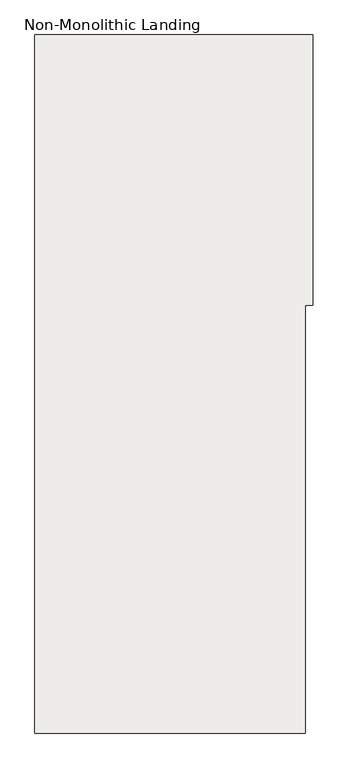
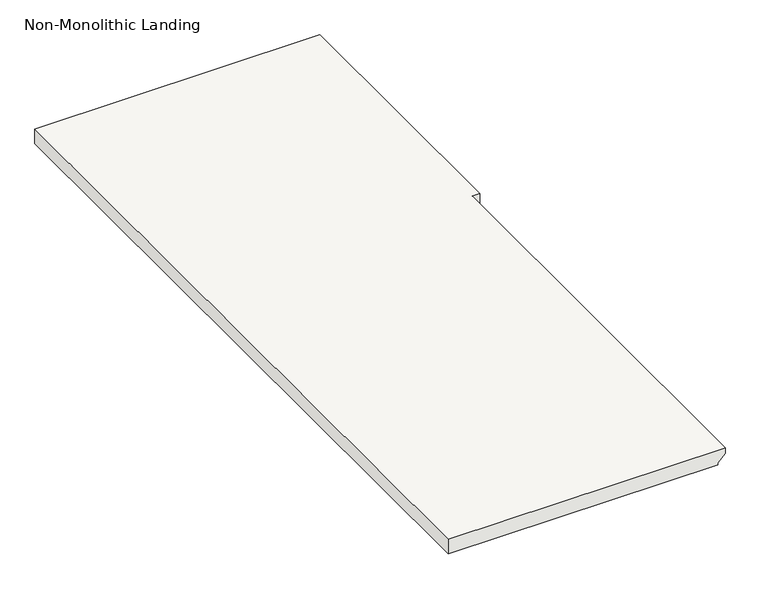
"""IFC4 building model written with IfcOpenShell, lengths in millimetres: slab geometry, Non-Monolithic Landing."""

from ifc_helpers import new_model, si_unit, origin, place, context, project, spatial, faceted_brep, source, transform, mapped, element, save


def non_monolithic_landing_b7697d37(model_context):
    return source(origin(), model_context, "Body", "Brep", [
        faceted_brep([(20207.1136801, 3970.8409313, 2546.35), (20181.7136801, 3970.8409313, 2520.95), (20181.7136801, 4885.2409313, 2520.95), (20207.1136801, 4885.2409313, 2546.35), (20207.1136801, 5418.6409313, 2565.4), (20232.5136801, 5418.6409313, 2565.4), (20232.5136801, 6333.0409313, 2565.4), (20207.1136801, 6333.0409313, 2565.4), (19292.7136801, 6333.0409313, 2565.4), (19292.7136801, 3970.8409313, 2565.4), (20207.1136801, 3970.8409313, 2565.4), (20181.7136801, 4885.2409313, 2514.6), (20181.7136801, 3970.8409313, 2514.6), (19292.7136801, 3970.8409313, 2514.6), (19292.7136801, 6333.0409313, 2514.6), (20207.1136801, 6333.0409313, 2514.6), (20232.5136801, 6333.0409313, 2514.6), (20232.5136801, 5418.6409313, 2514.6), (20207.1136801, 5418.6409313, 2514.6), (20207.1136801, 4885.2409313, 2514.6)], [[[0, 1, 2, 3]], [[4, 5, 6, 7, 8, 9, 10]], [[11, 12, 13, 14, 15, 16, 17, 18, 19]], [[12, 11, 2, 1]], [[11, 19, 3, 2]], [[4, 10, 0, 3, 19, 18]], [[5, 4, 18, 17]], [[6, 5, 17, 16]], [[7, 6, 16, 15]], [[8, 7, 15, 14]], [[9, 8, 14, 13]], [[10, 9, 13, 12, 1, 0]]]),
    ])


if __name__ == "__main__":
    model = new_model("IFC4")
    model_context = context("Model", 3, world=origin())
    ifc_project = project(units=[si_unit("LENGTHUNIT", "METRE", prefix="MILLI")], contexts=[model_context])
    site = spatial("IfcSite", under=ifc_project)
    building = spatial("IfcBuilding", under=site)
    placement = place(None, origin())
    non_monolithic_landing_shape = non_monolithic_landing_b7697d37(model_context)
    element("IfcSlab", 1, ObjectType="Non-Monolithic Landing", at=placement, inside=building, context=model_context, shape_type="MappedRepresentation", body=[
        mapped(non_monolithic_landing_shape, transform((0.0, 0.0, 0.0), x_axis=(1.0, 0.0, 0.0), y_axis=(0.0, 1.0, 0.0), z_axis=(0.0, 0.0, 1.0))),
    ])
    save(model, "model.ifc")
